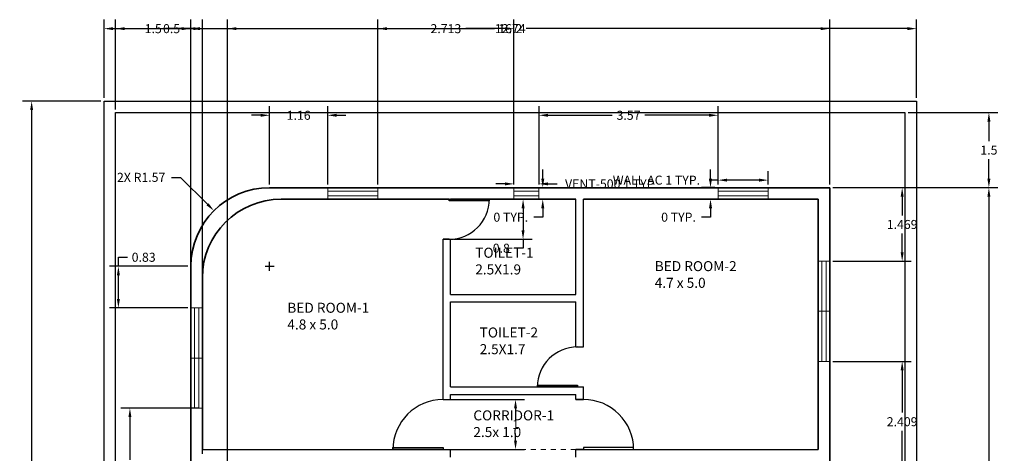
# Model space of a CAD drawing. Units: metres. Extents: x 2527.9 to 2558.5, y 2010.7 to 2033.1.
# Tile 3 of 3: x 2538.9 to 2558.5, y 2024.5 to 2033.1. Entities that reach past the tile are written whole.
import ezdxf

# ---------------------------------------------------------------- set-up
doc = ezdxf.new("R2010")
doc.units = ezdxf.units.M
doc.linetypes.add('ACAD_ISO02W100', pattern=[15, 12, -3])
for name, color, linetype, lineweight in [('A-ANNO-DIMS', 2, 'Continuous', 18), ('A-AREA-IDEN', 180, 'Continuous', 18), ('A-DOOR', 249, 'Continuous', 25), ('A-GLAZ', 249, 'Continuous', 18), ('A-WALL-OVHD', 6, 'ACAD_ISO02W100', 18), ('AC &V', 211, 'Continuous', 18), ('C-SITE-WALL', 110, 'Continuous', 30), ('INNER WALL', 109, 'Continuous', 30), ('OUTER WALL', 110, 'Continuous', 35)]:
    doc.layers.add(name, color=color, linetype=linetype, lineweight=lineweight)
doc.styles.get("Standard").update_dxf_attribs({"font": 'arial.ttf'})
doc.dimstyles.get("Standard").update_dxf_attribs({"dimtxt": 0.18, "dimasz": 0.18, "dimexe": 0.18, "dimexo": 0.0625, "dimgap": 0.09, "dimtad": 0, "dimtih": 1, "dimtoh": 1, "dimdec": 1, "dimzin": 0, "dimdsep": 46, "dimtxsty": 'Standard', "dimcen": 0.09, "dimadec": 0, "dimazin": 0, "dimtfac": 1, "dimtdec": 1, "dimtofl": 0, "dimtmove": 0, "dimatfit": 3, "dimfxl": 1, "dimtolj": 1, "dimtzin": 0, "dimarcsym": 0})

# ---------------------------------------------------------------- blocks, each defined once
blk = doc.blocks.new('*U2')
for p, q in [((0, 0), (0, -6)), ((40, 0), (40, -6))]:
    blk.add_line(p, q)
blk.add_lwpolyline([(0, 0), (0, 40), (1.75, 40), (1.75, 0)], close=True)
blk.add_arc((0, 0), 40, 0, 90)
blk = doc.blocks.new('*U4')
for p, q in [((0, 0), (0, 6)), ((40, 0), (40, 6))]:
    blk.add_line(p, q)
blk.add_lwpolyline([(0, 0), (0, -40), (1.75, -40), (1.75, 0)], close=True)
blk.add_arc((0, 0), 40, 270, 0)
blk = doc.blocks.new('*U3')
for p, q in [((-40, 0), (-40, 6)), ((0, 0), (0, 6))]:
    blk.add_line(p, q)
blk.add_lwpolyline([(0, 0), (0, -40), (-1.75, -40), (-1.75, 0)], close=True)
blk.add_arc((0, 0), 40, 180, 270)
blk = doc.blocks.new('WIN-2000-DOUBLE')
at = {"ltscale": 0.2}
for p, q in [((0, 0.23), (1, 0.23)), ((0, 0), (0, 0.23)), ((1, 0.23), (1, 0)), ((1, 0.23), (2, 0.23)), ((1, 0), (1, 0.23)), ((2, 0.23), (2, 0)), ((0, 0.16), (1, 0.16)), ((1, 0.07), (0, 0.07)), ((1, 0), (0, 0)), ((1, 0.16), (2, 0.16)), ((2, 0.07), (1, 0.07)), ((2, 0), (1, 0))]:
    blk.add_line(p, q, dxfattribs=at)
blk = doc.blocks.new('AC-WALL-1000')
at = {"ltscale": 0.2}
for p, q in [((0, 0.23), (1, 0.23)), ((0, 0), (0, 0.23)), ((1, 0.23), (1, 0)), ((0, 0.16), (1, 0.16)), ((1, 0.07), (0, 0.07)), ((1, 0), (0, 0))]:
    blk.add_line(p, q, dxfattribs=at)
blk = doc.blocks.new('VENT-500')
at = {"ltscale": 0.2}
for p, q in [((0, 0), (0, 0.5)), ((0.23, 0.5), (0, 0.5)), ((0.07, 0), (0.07, 0.5)), ((0.16, 0.5), (0.16, 0)), ((0.23, 0.5), (0.23, 0)), ((0.23, 0), (0, 0))]:
    blk.add_line(p, q, dxfattribs=at)
blk = doc.blocks.new('*D13')
at = {"layer": 'A-ANNO-DIMS', "color": 0, "lineweight": -2, "ltscale": 0.2, "transparency": 16777216}
for p, q in [((2552.796, 2029.847), (2552.796, 2030.115)), ((2553.796, 2029.847), (2553.796, 2030.115)), ((2552.796, 2029.935), (2552.616, 2029.935)), ((2553.616, 2029.935), (2552.976, 2029.935))]:
    blk.add_line(p, q, dxfattribs=at)
at = {"layer": 'A-ANNO-DIMS', "color": 0, "lineweight": -3, "ltscale": 0.2, "transparency": 16777216}
for points in [[(2552.976, 2029.965), (2552.976, 2029.905), (2552.796, 2029.935)], [(2553.616, 2029.965), (2553.616, 2029.905), (2553.796, 2029.935)]]:
    blk.add_solid(points, dxfattribs=at)
at = {"layer": 'Defpoints', "color": 0, "lineweight": -3, "ltscale": 0.2, "transparency": 16777216}
for p in [(2552.796, 2029.935), (2552.796, 2029.785), (2553.796, 2029.785)]:
    blk.add_point(p, dxfattribs=at)
at = {"layer": 'A-ANNO-DIMS', "color": 0, "ltscale": 0.2, "transparency": 16777216, "insert": (2551.567, 2029.935), "char_height": 0.18, "attachment_point": 5}
blk.add_mtext('\\A1;WALL AC 1 TYP.', dxfattribs=at)
blk = doc.blocks.new('*D14')
at = {"layer": 'A-ANNO-DIMS', "color": 0, "lineweight": -2, "ltscale": 0.2, "transparency": 16777216}
for p, q in [((2552.646, 2029.965), (2552.646, 2030.145)), ((2552.734, 2029.785), (2552.466, 2029.785)), ((2552.734, 2029.555), (2552.466, 2029.555)), ((2552.646, 2029.375), (2552.646, 2029.195)), ((2552.646, 2029.195), (2552.466, 2029.195))]:
    blk.add_line(p, q, dxfattribs=at)
at = {"layer": 'A-ANNO-DIMS', "color": 0, "lineweight": -3, "ltscale": 0.2, "transparency": 16777216}
for points in [[(2552.616, 2029.965), (2552.676, 2029.965), (2552.646, 2029.785)], [(2552.616, 2029.375), (2552.676, 2029.375), (2552.646, 2029.555)]]:
    blk.add_solid(points, dxfattribs=at)
at = {"layer": 'Defpoints', "color": 0, "lineweight": -3, "ltscale": 0.2, "transparency": 16777216}
for p in [(2552.796, 2029.785), (2552.646, 2029.555), (2552.796, 2029.555)]:
    blk.add_point(p, dxfattribs=at)
at = {"layer": 'A-ANNO-DIMS', "color": 0, "ltscale": 0.2, "transparency": 16777216, "insert": (2552.008, 2029.195), "char_height": 0.18, "attachment_point": 5}
blk.add_mtext('\\A1;0 TYP.', dxfattribs=at)
blk = doc.blocks.new('*D15')
at = {"layer": 'A-ANNO-DIMS', "color": 0, "lineweight": -2, "ltscale": 0.2, "transparency": 16777216}
for p, q in [((2548.726, 2029.847), (2548.726, 2030.04)), ((2549.226, 2029.847), (2549.226, 2030.04)), ((2548.546, 2029.86), (2548.366, 2029.86)), ((2549.406, 2029.86), (2549.586, 2029.86))]:
    blk.add_line(p, q, dxfattribs=at)
at = {"layer": 'A-ANNO-DIMS', "color": 0, "lineweight": -3, "ltscale": 0.2, "transparency": 16777216}
for points in [[(2548.546, 2029.89), (2548.546, 2029.83), (2548.726, 2029.86)], [(2549.406, 2029.89), (2549.406, 2029.83), (2549.226, 2029.86)]]:
    blk.add_solid(points, dxfattribs=at)
at = {"layer": 'Defpoints', "color": 0, "lineweight": -3, "ltscale": 0.2, "transparency": 16777216}
for p in [(2548.726, 2029.785), (2549.226, 2029.86), (2549.226, 2029.785)]:
    blk.add_point(p, dxfattribs=at)
at = {"layer": 'A-ANNO-DIMS', "color": 0, "ltscale": 0.2, "transparency": 16777216, "insert": (2550.671, 2029.86), "char_height": 0.18, "attachment_point": 5}
blk.add_mtext('\\A1;VENT-500 1 TYP.', dxfattribs=at)
blk = doc.blocks.new('*D16')
at = {"layer": 'A-ANNO-DIMS', "color": 0, "lineweight": -2, "ltscale": 0.2, "transparency": 16777216}
for p, q in [((2549.301, 2029.965), (2549.301, 2030.145)), ((2549.288, 2029.785), (2549.481, 2029.785)), ((2549.288, 2029.555), (2549.481, 2029.555)), ((2549.301, 2029.375), (2549.301, 2029.195)), ((2549.301, 2029.195), (2549.121, 2029.195))]:
    blk.add_line(p, q, dxfattribs=at)
at = {"layer": 'A-ANNO-DIMS', "color": 0, "lineweight": -3, "ltscale": 0.2, "transparency": 16777216}
for points in [[(2549.271, 2029.965), (2549.331, 2029.965), (2549.301, 2029.785)], [(2549.271, 2029.375), (2549.331, 2029.375), (2549.301, 2029.555)]]:
    blk.add_solid(points, dxfattribs=at)
at = {"layer": 'Defpoints', "color": 0, "lineweight": -3, "ltscale": 0.2, "transparency": 16777216}
for p in [(2549.226, 2029.785), (2549.226, 2029.555), (2549.301, 2029.555)]:
    blk.add_point(p, dxfattribs=at)
at = {"layer": 'A-ANNO-DIMS', "color": 0, "ltscale": 0.2, "transparency": 16777216, "insert": (2548.663, 2029.195), "char_height": 0.18, "attachment_point": 5}
blk.add_mtext('\\A1;0 TYP.', dxfattribs=at)
blk = doc.blocks.new('*D17')
at = {"layer": 'A-ANNO-DIMS', "color": 0, "lineweight": -2, "ltscale": 0.2, "transparency": 16777216}
for p, q in [((2540.553, 2031.577), (2540.553, 2033.14)), ((2556.753, 2031.577), (2556.753, 2033.14)), ((2540.733, 2032.96), (2548.339, 2032.96)), ((2556.573, 2032.96), (2548.968, 2032.96))]:
    blk.add_line(p, q, dxfattribs=at)
at = {"layer": 'A-ANNO-DIMS', "color": 0, "lineweight": -3, "ltscale": 0.2, "transparency": 16777216}
for points in [[(2540.733, 2032.99), (2540.733, 2032.93), (2540.553, 2032.96)], [(2556.573, 2032.99), (2556.573, 2032.93), (2556.753, 2032.96)]]:
    blk.add_solid(points, dxfattribs=at)
at = {"layer": 'Defpoints', "color": 0, "lineweight": -3, "ltscale": 0.2, "transparency": 16777216}
for p in [(2556.753, 2032.96), (2540.553, 2031.515), (2556.753, 2031.515)]:
    blk.add_point(p, dxfattribs=at)
at = {"layer": 'A-ANNO-DIMS', "color": 0, "ltscale": 0.2, "transparency": 16777216, "insert": (2548.653, 2032.96), "char_height": 0.18, "attachment_point": 5}
blk.add_mtext('\\A1;16.2', dxfattribs=at)
blk = doc.blocks.new('*D18')
at = {"layer": 'A-ANNO-DIMS', "color": 0, "lineweight": -2, "ltscale": 0.2, "transparency": 16777216}
for p, q in [((2540.491, 2031.515), (2538.928, 2031.515)), ((2539.108, 2031.335), (2539.108, 2022.096)), ((2539.108, 2012.495), (2539.108, 2021.733)), ((2540.491, 2012.315), (2538.928, 2012.315))]:
    blk.add_line(p, q, dxfattribs=at)
at = {"layer": 'A-ANNO-DIMS', "color": 0, "lineweight": -3, "ltscale": 0.2, "transparency": 16777216}
for points in [[(2539.078, 2031.335), (2539.138, 2031.335), (2539.108, 2031.515)], [(2539.078, 2012.495), (2539.138, 2012.495), (2539.108, 2012.315)]]:
    blk.add_solid(points, dxfattribs=at)
at = {"layer": 'Defpoints', "color": 0, "lineweight": -3, "ltscale": 0.2, "transparency": 16777216}
for p in [(2539.108, 2031.515), (2540.553, 2031.515), (2540.553, 2012.315)]:
    blk.add_point(p, dxfattribs=at)
at = {"layer": 'A-ANNO-DIMS', "color": 0, "ltscale": 0.2, "transparency": 16777216, "insert": (2539.108, 2021.915), "char_height": 0.18, "attachment_point": 5}
blk.add_mtext('\\A1;19.2', dxfattribs=at)
blk = doc.blocks.new('*D19')
at = {"layer": 'A-ANNO-DIMS', "color": 0, "lineweight": -2, "ltscale": 0.2, "transparency": 16777216}
for p, q in [((2542.283, 2028.277), (2542.283, 2033.14)), ((2555.023, 2029.847), (2555.023, 2033.14)), ((2542.463, 2032.96), (2548.268, 2032.96)), ((2554.843, 2032.96), (2549.038, 2032.96))]:
    blk.add_line(p, q, dxfattribs=at)
at = {"layer": 'A-ANNO-DIMS', "color": 0, "lineweight": -3, "ltscale": 0.2, "transparency": 16777216}
for points in [[(2542.463, 2032.99), (2542.463, 2032.93), (2542.283, 2032.96)], [(2554.843, 2032.99), (2554.843, 2032.93), (2555.023, 2032.96)]]:
    blk.add_solid(points, dxfattribs=at)
at = {"layer": 'Defpoints', "color": 0, "lineweight": -3, "ltscale": 0.2, "transparency": 16777216}
for p in [(2555.023, 2032.96), (2555.023, 2029.785), (2542.283, 2028.215)]:
    blk.add_point(p, dxfattribs=at)
at = {"layer": 'A-ANNO-DIMS', "color": 0, "ltscale": 0.2, "transparency": 16777216, "insert": (2548.653, 2032.96), "char_height": 0.18, "attachment_point": 5}
blk.add_mtext('\\A1;12.74', dxfattribs=at)
blk = doc.blocks.new('*D20')
at = {"layer": 'A-ANNO-DIMS', "color": 0, "lineweight": -2, "ltscale": 0.2, "transparency": 16777216}
for p, q in [((2555.086, 2029.785), (2558.378, 2029.785)), ((2558.198, 2029.605), (2558.198, 2022.602)), ((2558.198, 2015.235), (2558.198, 2022.238)), ((2555.086, 2015.055), (2558.378, 2015.055))]:
    blk.add_line(p, q, dxfattribs=at)
at = {"layer": 'A-ANNO-DIMS', "color": 0, "lineweight": -3, "ltscale": 0.2, "transparency": 16777216}
for points in [[(2558.168, 2029.605), (2558.228, 2029.605), (2558.198, 2029.785)], [(2558.168, 2015.235), (2558.228, 2015.235), (2558.198, 2015.055)]]:
    blk.add_solid(points, dxfattribs=at)
at = {"layer": 'Defpoints', "color": 0, "lineweight": -3, "ltscale": 0.2, "transparency": 16777216}
for p in [(2555.023, 2029.785), (2558.198, 2029.785), (2555.023, 2015.055)]:
    blk.add_point(p, dxfattribs=at)
at = {"layer": 'A-ANNO-DIMS', "color": 0, "ltscale": 0.2, "transparency": 16777216, "insert": (2558.198, 2022.42), "char_height": 0.18, "attachment_point": 5}
blk.add_mtext('\\A1;14.73', dxfattribs=at)
blk = doc.blocks.new('*D21')
at = {"layer": 'A-ANNO-DIMS', "color": 0, "lineweight": -2, "ltscale": 0.2, "transparency": 16777216}
for p, q in [((2540.783, 2031.347), (2540.783, 2033.14)), ((2542.283, 2028.277), (2542.283, 2033.14)), ((2540.963, 2032.96), (2541.287, 2032.96)), ((2542.103, 2032.96), (2541.779, 2032.96))]:
    blk.add_line(p, q, dxfattribs=at)
at = {"layer": 'A-ANNO-DIMS', "color": 0, "lineweight": -3, "ltscale": 0.2, "transparency": 16777216}
for points in [[(2540.963, 2032.99), (2540.963, 2032.93), (2540.783, 2032.96)], [(2542.103, 2032.99), (2542.103, 2032.93), (2542.283, 2032.96)]]:
    blk.add_solid(points, dxfattribs=at)
at = {"layer": 'Defpoints', "color": 0, "lineweight": -3, "ltscale": 0.2, "transparency": 16777216}
for p in [(2542.283, 2032.96), (2540.783, 2031.285), (2542.283, 2028.215)]:
    blk.add_point(p, dxfattribs=at)
at = {"layer": 'A-ANNO-DIMS', "color": 0, "ltscale": 0.2, "transparency": 16777216, "insert": (2541.533, 2032.96), "char_height": 0.18, "attachment_point": 5}
blk.add_mtext('\\A1;1.5', dxfattribs=at)
blk = doc.blocks.new('*D22')
at = {"layer": 'A-ANNO-DIMS', "color": 0, "lineweight": -2, "ltscale": 0.2, "transparency": 16777216}
for p, q in [((2556.586, 2031.285), (2558.378, 2031.285)), ((2558.198, 2031.105), (2558.198, 2030.716)), ((2558.198, 2029.965), (2558.198, 2030.353)), ((2555.086, 2029.785), (2558.378, 2029.785))]:
    blk.add_line(p, q, dxfattribs=at)
at = {"layer": 'A-ANNO-DIMS', "color": 0, "lineweight": -3, "ltscale": 0.2, "transparency": 16777216}
for points in [[(2558.168, 2031.105), (2558.228, 2031.105), (2558.198, 2031.285)], [(2558.168, 2029.965), (2558.228, 2029.965), (2558.198, 2029.785)]]:
    blk.add_solid(points, dxfattribs=at)
at = {"layer": 'Defpoints', "color": 0, "lineweight": -3, "ltscale": 0.2, "transparency": 16777216}
for p in [(2556.523, 2031.285), (2558.198, 2031.285), (2555.023, 2029.785)]:
    blk.add_point(p, dxfattribs=at)
at = {"layer": 'A-ANNO-DIMS', "color": 0, "ltscale": 0.2, "transparency": 16777216, "insert": (2558.198, 2030.535), "char_height": 0.18, "attachment_point": 5}
blk.add_mtext('\\A1;1.5', dxfattribs=at)
blk = doc.blocks.new('*D50')
at = {"layer": 'A-ANNO-DIMS', "color": 0, "lineweight": -2, "ltscale": 0.2, "transparency": 16777216}
for p, q in [((2543.853, 2029.847), (2543.853, 2031.41)), ((2545.013, 2029.847), (2545.013, 2031.41)), ((2543.673, 2031.23), (2543.493, 2031.23)), ((2545.193, 2031.23), (2545.373, 2031.23))]:
    blk.add_line(p, q, dxfattribs=at)
at = {"layer": 'A-ANNO-DIMS', "color": 0, "lineweight": -3, "ltscale": 0.2, "transparency": 16777216}
for points in [[(2543.673, 2031.26), (2543.673, 2031.2), (2543.853, 2031.23)], [(2545.193, 2031.26), (2545.193, 2031.2), (2545.013, 2031.23)]]:
    blk.add_solid(points, dxfattribs=at)
at = {"layer": 'Defpoints', "color": 0, "lineweight": -3, "ltscale": 0.2, "transparency": 16777216}
for p in [(2545.013, 2031.23), (2543.853, 2029.785), (2545.013, 2029.785)]:
    blk.add_point(p, dxfattribs=at)
at = {"layer": 'A-ANNO-DIMS', "color": 0, "ltscale": 0.2, "transparency": 16777216, "insert": (2544.433, 2031.23), "char_height": 0.18, "attachment_point": 5}
blk.add_mtext('\\A1;1.16', dxfattribs=at)
blk = doc.blocks.new('*D51')
at = {"layer": 'A-ANNO-DIMS', "color": 0, "lineweight": -2, "ltscale": 0.2, "transparency": 16777216}
for p, q in [((2546.013, 2029.847), (2546.013, 2033.14)), ((2548.726, 2029.847), (2548.726, 2033.14)), ((2546.193, 2032.96), (2546.974, 2032.96)), ((2548.546, 2032.96), (2547.765, 2032.96))]:
    blk.add_line(p, q, dxfattribs=at)
at = {"layer": 'A-ANNO-DIMS', "color": 0, "lineweight": -3, "ltscale": 0.2, "transparency": 16777216}
for points in [[(2546.193, 2032.99), (2546.193, 2032.93), (2546.013, 2032.96)], [(2548.546, 2032.99), (2548.546, 2032.93), (2548.726, 2032.96)]]:
    blk.add_solid(points, dxfattribs=at)
at = {"layer": 'Defpoints', "color": 0, "lineweight": -3, "ltscale": 0.2, "transparency": 16777216}
for p in [(2548.726, 2032.96), (2546.013, 2029.785), (2548.726, 2029.785)]:
    blk.add_point(p, dxfattribs=at)
at = {"layer": 'A-ANNO-DIMS', "color": 0, "ltscale": 0.2, "transparency": 16777216, "insert": (2547.369, 2032.96), "char_height": 0.18, "attachment_point": 5}
blk.add_mtext('\\A1;2.713', dxfattribs=at)
blk = doc.blocks.new('*D52')
at = {"layer": 'A-ANNO-DIMS', "color": 0, "lineweight": -2, "ltscale": 0.2, "transparency": 16777216}
for p, q in [((2549.226, 2029.847), (2549.226, 2031.41)), ((2552.796, 2029.847), (2552.796, 2031.41)), ((2549.406, 2031.23), (2550.687, 2031.23)), ((2552.616, 2031.23), (2551.335, 2031.23))]:
    blk.add_line(p, q, dxfattribs=at)
at = {"layer": 'A-ANNO-DIMS', "color": 0, "lineweight": -3, "ltscale": 0.2, "transparency": 16777216}
for points in [[(2549.406, 2031.26), (2549.406, 2031.2), (2549.226, 2031.23)], [(2552.616, 2031.26), (2552.616, 2031.2), (2552.796, 2031.23)]]:
    blk.add_solid(points, dxfattribs=at)
at = {"layer": 'Defpoints', "color": 0, "lineweight": -3, "ltscale": 0.2, "transparency": 16777216}
for p in [(2552.796, 2031.23), (2549.226, 2029.785), (2552.796, 2029.785)]:
    blk.add_point(p, dxfattribs=at)
at = {"layer": 'A-ANNO-DIMS', "color": 0, "ltscale": 0.2, "transparency": 16777216, "insert": (2551.011, 2031.23), "char_height": 0.18, "attachment_point": 5}
blk.add_mtext('\\A1;3.57', dxfattribs=at)
blk = doc.blocks.new('*D53')
at = {"layer": 'A-ANNO-DIMS', "color": 0, "lineweight": -2, "ltscale": 0.2, "transparency": 16777216}
for p, q in [((2555.086, 2029.785), (2556.648, 2029.785)), ((2556.468, 2029.605), (2556.468, 2029.232)), ((2556.468, 2028.496), (2556.468, 2028.868)), ((2555.086, 2028.316), (2556.648, 2028.316))]:
    blk.add_line(p, q, dxfattribs=at)
at = {"layer": 'A-ANNO-DIMS', "color": 0, "lineweight": -3, "ltscale": 0.2, "transparency": 16777216}
for points in [[(2556.438, 2029.605), (2556.498, 2029.605), (2556.468, 2029.785)], [(2556.438, 2028.496), (2556.498, 2028.496), (2556.468, 2028.316)]]:
    blk.add_solid(points, dxfattribs=at)
at = {"layer": 'Defpoints', "color": 0, "lineweight": -3, "ltscale": 0.2, "transparency": 16777216}
for p in [(2555.023, 2029.785), (2555.023, 2028.316), (2556.468, 2028.316)]:
    blk.add_point(p, dxfattribs=at)
at = {"layer": 'A-ANNO-DIMS', "color": 0, "ltscale": 0.2, "transparency": 16777216, "insert": (2556.468, 2029.05), "char_height": 0.18, "attachment_point": 5}
blk.add_mtext('\\A1;1.469', dxfattribs=at)
blk = doc.blocks.new('*D54')
at = {"layer": 'A-ANNO-DIMS', "color": 0, "lineweight": -2, "ltscale": 0.2, "transparency": 16777216}
for p, q in [((2555.086, 2026.316), (2556.648, 2026.316)), ((2556.468, 2026.136), (2556.468, 2025.293)), ((2556.468, 2024.087), (2556.468, 2024.929)), ((2555.086, 2023.907), (2556.648, 2023.907))]:
    blk.add_line(p, q, dxfattribs=at)
at = {"layer": 'A-ANNO-DIMS', "color": 0, "lineweight": -3, "ltscale": 0.2, "transparency": 16777216}
for points in [[(2556.438, 2026.136), (2556.498, 2026.136), (2556.468, 2026.316)], [(2556.438, 2024.087), (2556.498, 2024.087), (2556.468, 2023.907)]]:
    blk.add_solid(points, dxfattribs=at)
at = {"layer": 'Defpoints', "color": 0, "lineweight": -3, "ltscale": 0.2, "transparency": 16777216}
for p in [(2555.023, 2026.316), (2555.023, 2023.907), (2556.468, 2023.907)]:
    blk.add_point(p, dxfattribs=at)
at = {"layer": 'A-ANNO-DIMS', "color": 0, "ltscale": 0.2, "transparency": 16777216, "insert": (2556.468, 2025.111), "char_height": 0.18, "attachment_point": 5}
blk.add_mtext('\\A1;2.409', dxfattribs=at)
blk = doc.blocks.new('*D57')
at = {"layer": 'A-ANNO-DIMS', "color": 0, "lineweight": -2, "ltscale": 0.2, "transparency": 16777216}
for p, q in [((2540.838, 2028.215), (2540.838, 2028.395)), ((2540.838, 2028.395), (2541.018, 2028.395)), ((2542.221, 2028.215), (2540.658, 2028.215)), ((2540.838, 2027.563), (2540.838, 2028.035)), ((2542.221, 2027.383), (2540.658, 2027.383))]:
    blk.add_line(p, q, dxfattribs=at)
at = {"layer": 'A-ANNO-DIMS', "color": 0, "lineweight": -3, "ltscale": 0.2, "transparency": 16777216}
for points in [[(2540.808, 2028.035), (2540.868, 2028.035), (2540.838, 2028.215)], [(2540.808, 2027.563), (2540.868, 2027.563), (2540.838, 2027.383)]]:
    blk.add_solid(points, dxfattribs=at)
at = {"layer": 'Defpoints', "color": 0, "lineweight": -3, "ltscale": 0.2, "transparency": 16777216}
for p in [(2540.838, 2028.215), (2542.283, 2028.215), (2542.283, 2027.383)]:
    blk.add_point(p, dxfattribs=at)
at = {"layer": 'A-ANNO-DIMS', "color": 0, "ltscale": 0.2, "transparency": 16777216, "insert": (2541.342, 2028.395), "char_height": 0.18, "attachment_point": 5}
blk.add_mtext('\\A1;0.83', dxfattribs=at)
blk = doc.blocks.new('*D58')
at = {"layer": 'A-ANNO-DIMS', "color": 0, "lineweight": -2, "ltscale": 0.2, "transparency": 16777216}
for p, q in [((2542.451, 2025.383), (2540.888, 2025.383)), ((2541.068, 2025.203), (2541.068, 2024.351)), ((2541.068, 2023.139), (2541.068, 2023.991)), ((2542.451, 2022.959), (2540.888, 2022.959))]:
    blk.add_line(p, q, dxfattribs=at)
at = {"layer": 'A-ANNO-DIMS', "color": 0, "lineweight": -3, "ltscale": 0.2, "transparency": 16777216}
for points in [[(2541.038, 2025.203), (2541.098, 2025.203), (2541.068, 2025.383)], [(2541.038, 2023.139), (2541.098, 2023.139), (2541.068, 2022.959)]]:
    blk.add_solid(points, dxfattribs=at)
at = {"layer": 'Defpoints', "color": 0, "lineweight": -3, "ltscale": 0.2, "transparency": 16777216}
for p in [(2541.068, 2025.383), (2542.513, 2025.383), (2542.513, 2022.959)]:
    blk.add_point(p, dxfattribs=at)
at = {"layer": 'A-ANNO-DIMS', "color": 0, "ltscale": 0.2, "transparency": 16777216, "insert": (2541.068, 2024.171), "char_height": 0.18, "attachment_point": 5}
blk.add_mtext('\\A1;2.42', dxfattribs=at)
blk = doc.blocks.new('*D63')
at = {"layer": 'A-ANNO-DIMS', "color": 0, "lineweight": -2, "ltscale": 0.2, "transparency": 16777216}
for p, q in [((2547.376, 2025.555), (2548.938, 2025.555)), ((2548.758, 2025.375), (2548.758, 2025.235)), ((2548.758, 2024.735), (2548.758, 2024.874)), ((2547.376, 2024.555), (2548.938, 2024.555))]:
    blk.add_line(p, q, dxfattribs=at)
at = {"layer": 'A-ANNO-DIMS', "color": 0, "lineweight": -3, "ltscale": 0.2, "transparency": 16777216}
for points in [[(2548.728, 2025.375), (2548.788, 2025.375), (2548.758, 2025.555)], [(2548.728, 2024.735), (2548.788, 2024.735), (2548.758, 2024.555)]]:
    blk.add_solid(points, dxfattribs=at)
at = {"layer": 'Defpoints', "color": 0, "lineweight": -3, "ltscale": 0.2, "transparency": 16777216}
for p in [(2547.313, 2025.555), (2547.313, 2024.555), (2548.758, 2024.555)]:
    blk.add_point(p, dxfattribs=at)
at = {"layer": 'A-ANNO-DIMS', "color": 0, "ltscale": 0.2, "transparency": 16777216, "insert": (2548.758, 2025.055), "char_height": 0.18, "attachment_point": 5}
blk.add_mtext('\\A1;1', dxfattribs=at)
blk = doc.blocks.new('*D64')
at = {"layer": 'A-ANNO-DIMS', "color": 0, "lineweight": -2, "ltscale": 0.2, "transparency": 16777216}
for p, q in [((2547.526, 2029.555), (2549.088, 2029.555)), ((2548.908, 2029.375), (2548.908, 2028.935)), ((2547.526, 2028.755), (2549.088, 2028.755)), ((2548.908, 2028.755), (2548.908, 2028.575)), ((2548.908, 2028.575), (2548.728, 2028.575))]:
    blk.add_line(p, q, dxfattribs=at)
at = {"layer": 'A-ANNO-DIMS', "color": 0, "lineweight": -3, "ltscale": 0.2, "transparency": 16777216}
for points in [[(2548.878, 2029.375), (2548.938, 2029.375), (2548.908, 2029.555)], [(2548.878, 2028.935), (2548.938, 2028.935), (2548.908, 2028.755)]]:
    blk.add_solid(points, dxfattribs=at)
at = {"layer": 'Defpoints', "color": 0, "lineweight": -3, "ltscale": 0.2, "transparency": 16777216}
for p in [(2547.463, 2029.555), (2547.463, 2028.755), (2548.908, 2028.755)]:
    blk.add_point(p, dxfattribs=at)
at = {"layer": 'A-ANNO-DIMS', "color": 0, "ltscale": 0.2, "transparency": 16777216, "insert": (2548.474, 2028.575), "char_height": 0.18, "attachment_point": 5}
blk.add_mtext('\\A1;0.8', dxfattribs=at)
blk = doc.blocks.new('*D65')
at = {"layer": 'A-ANNO-DIMS', "color": 0, "lineweight": -2, "ltscale": 0.2, "transparency": 16777216}
for p, q in [((2542.513, 2024.467), (2542.513, 2033.14)), ((2543.013, 2023.967), (2543.013, 2033.14)), ((2542.333, 2032.96), (2542.153, 2032.96)), ((2543.193, 2032.96), (2543.373, 2032.96))]:
    blk.add_line(p, q, dxfattribs=at)
at = {"layer": 'A-ANNO-DIMS', "color": 0, "lineweight": -3, "ltscale": 0.2, "transparency": 16777216}
for points in [[(2542.333, 2032.99), (2542.333, 2032.93), (2542.513, 2032.96)], [(2543.193, 2032.99), (2543.193, 2032.93), (2543.013, 2032.96)]]:
    blk.add_solid(points, dxfattribs=at)
at = {"layer": 'Defpoints', "color": 0, "lineweight": -3, "ltscale": 0.2, "transparency": 16777216}
for p in [(2542.513, 2032.96), (2542.513, 2024.405), (2543.013, 2023.905)]:
    blk.add_point(p, dxfattribs=at)
at = {"layer": 'A-ANNO-DIMS', "color": 0, "ltscale": 0.2, "transparency": 16777216, "insert": (2541.899, 2032.96), "char_height": 0.18, "attachment_point": 5}
blk.add_mtext('\\A1;0.5', dxfattribs=at)
blk = doc.blocks.new('*D66')
at = {"layer": 'A-ANNO-DIMS', "color": 0, "lineweight": -2, "ltscale": 0.2, "transparency": 16777216}
for p, q in [((2541.897, 2029.991), (2542.077, 2029.991)), ((2542.077, 2029.991), (2542.616, 2029.452)), ((2543.763, 2028.215), (2543.943, 2028.215)), ((2543.853, 2028.125), (2543.853, 2028.305))]:
    blk.add_line(p, q, dxfattribs=at)
at = {"layer": 'A-ANNO-DIMS', "color": 0, "lineweight": -3, "ltscale": 0.2, "transparency": 16777216}
blk.add_solid([(2542.637, 2029.473), (2542.595, 2029.431), (2542.743, 2029.325)], dxfattribs=at)
at = {"layer": 'Defpoints', "color": 0, "lineweight": -3, "ltscale": 0.2, "transparency": 16777216}
for p in [(2542.743, 2029.325), (2543.853, 2028.215)]:
    blk.add_point(p, dxfattribs=at)
at = {"layer": 'A-ANNO-DIMS', "color": 0, "ltscale": 0.2, "transparency": 16777216, "insert": (2541.292, 2029.991), "char_height": 0.18, "attachment_point": 5}
blk.add_mtext('\\A1;2X R1.57', dxfattribs=at)

msp = doc.modelspace()

# ---------------------------------------------------------------- linework, layer by layer
at = {"layer": 'A-WALL-OVHD', "ltscale": 0.002}
msp.add_line((2547.4633, 2024.5545), (2549.9633, 2024.5545), dxfattribs=at)
at = {"layer": 'C-SITE-WALL'}
for p, q in [((2540.5533, 2031.5145), (2556.7533, 2031.5145)), ((2540.7833, 2031.2845), (2556.5233, 2031.2845))]:
    msp.add_line(p, q, dxfattribs=at)
for points in [[(2548.0644, 2012.3145), (2540.5533, 2012.3145), (2540.5533, 2031.5145)], [(2556.7533, 2031.5145), (2556.7533, 2012.3145), (2551.0644, 2012.3145)], [(2548.0644, 2012.5445), (2540.7833, 2012.5445), (2540.7833, 2031.2845)], [(2556.5233, 2031.2845), (2556.5233, 2012.5445), (2551.0644, 2012.5445)]]:
    msp.add_lwpolyline(points, dxfattribs=at)
at = {"layer": 'INNER WALL'}
for p, q in [((2547.3133, 2029.5545), (2547.4633, 2029.5545)), ((2549.9633, 2027.6545), (2549.9633, 2029.5545)), ((2550.1133, 2026.6045), (2550.1133, 2029.5545)), ((2547.3133, 2028.7545), (2547.4633, 2028.7545)), ((2547.3133, 2025.5545), (2547.3133, 2028.7545)), ((2547.4633, 2027.6545), (2547.4633, 2028.7545)), ((2547.4633, 2027.6545), (2549.9633, 2027.6545)), ((2547.4633, 2027.5045), (2549.9633, 2027.5045)), ((2547.4633, 2025.8045), (2547.4633, 2027.5045)), ((2549.9633, 2026.6045), (2549.9633, 2027.5045)), ((2549.9633, 2026.6045), (2550.1133, 2026.6045)), ((2547.4633, 2025.8045), (2549.9633, 2025.8045)), ((2549.9633, 2025.8045), (2550.1133, 2025.8045)), ((2550.1133, 2025.5545), (2550.1133, 2025.8045)), ((2547.4633, 2025.6545), (2549.9633, 2025.6545)), ((2547.4633, 2025.5545), (2547.4633, 2025.6545)), ((2549.9633, 2025.5545), (2549.9633, 2025.6545)), ((2549.9633, 2025.5545), (2549.9633, 2025.6545)), ((2547.3133, 2025.5545), (2547.4633, 2025.5545)), ((2549.9633, 2025.5545), (2550.1133, 2025.5545)), ((2542.5133, 2024.5545), (2547.3133, 2024.5545)), ((2547.3133, 2024.5545), (2547.4633, 2024.5545)), ((2547.4633, 2024.4045), (2547.4633, 2024.5545)), ((2549.9633, 2024.5545), (2550.1133, 2024.5545)), ((2549.9633, 2024.4045), (2549.9633, 2024.5545)), ((2550.1133, 2024.5545), (2554.7933, 2024.5545))]:
    msp.add_line(p, q, dxfattribs=at)
at = {"layer": 'OUTER WALL'}
for p, q in [((2543.8533, 2029.7845), (2555.0233, 2029.7845)), ((2555.0233, 2029.7845), (2555.0233, 2015.0545)), ((2544.0833, 2029.5545), (2547.3133, 2029.5545)), ((2547.4633, 2029.5545), (2549.9633, 2029.5545)), ((2550.1133, 2029.5545), (2554.7933, 2029.5545)), ((2554.7933, 2029.5545), (2554.7933, 2024.5545)), ((2542.2833, 2015.5245), (2542.2833, 2028.2145)), ((2542.5133, 2024.5545), (2542.5133, 2027.9845))]:
    msp.add_line(p, q, dxfattribs=at)
for centre in [(2543.8533, 2028.2145), (2544.0833, 2027.9845)]:
    msp.add_arc(centre, 1.57, 90, 180, dxfattribs=at)

# ---------------------------------------------------------------- block references
at = {"layer": 'A-DOOR'}
for name, p, xscale, yscale, zscale, rotation in [('*U2', (2547.4333, 2029.5545), 0.0199999999999985, 0.0199999999999985, 0.0199999999999985, 270), ('*U2', (2549.9933, 2025.8045), 0.0199999999999985, 0.0199999999999985, 0.0199999999999985, 89.99999999999999), ('*U3', (2547.3133, 2024.5545), 0.0249999999999996, 0.0249999999999996, 0.0249999999999996, 270), ('*U4', (2550.1133, 2024.5545), 0.0249999999999996, 0.0249999999999996, 0.0249999999999996, 89.99999999999999)]:
    msp.add_blockref(name, p, dxfattribs=dict(at, xscale=xscale, yscale=yscale, zscale=zscale, rotation=rotation))
at = {"layer": 'A-GLAZ'}
for p, rotation in [((2555.0233, 2026.3157), 89.99999999998612), ((2542.5133, 2025.3831), 90.00000000002422)]:
    msp.add_blockref('WIN-2000-DOUBLE', p, dxfattribs=dict(at, rotation=rotation))
at = {"layer": 'AC &V'}
msp.add_blockref('AC-WALL-1000', (2545.0129, 2029.5545), dxfattribs=at)
for name, p, rotation in [('VENT-500', (2548.7258, 2029.7845), 270.0000000002778), ('AC-WALL-1000', (2553.7962, 2029.7845), 180)]:
    msp.add_blockref(name, p, dxfattribs=dict(at, rotation=rotation))

# ---------------------------------------------------------------- texts
at = {"layer": 'A-AREA-IDEN', "char_height": 0.2, "attachment_point": 1}
for s, width, insert in [('TOILET-1 2.5X1.9', 1.31727, (2547.9548, 2028.5853)), ('BED ROOM-2   4.7 x 5.0', 1.785754, (2551.5337, 2028.3176)), ('BED ROOM-1   4.8 x 5.0', 1.809794, (2544.2069, 2027.4863)), ('TOILET-2 2.5X1.7', 1.31727, (2548.0427, 2026.9929)), ('CORRIDOR-1   2.5x 1.0', 1.770765, (2547.9162, 2025.3377))]:
    msp.add_mtext_dynamic_manual_height_columns(s, width=width, gutter_width=12.5, heights=[0], dxfattribs=dict(at, insert=insert))

# ---------------------------------------------------------------- dimensions: what is measured, and where the dimension line sits
at = {"layer": 'A-ANNO-DIMS', "ltscale": 0.2}
for base, p1, p2, override, picture, middle in [((2556.7533, 2032.9595), (2540.5533, 2031.5145), (2556.7533, 2031.5145), {"dimdec": 1, "dimlfac": 1, "dimrnd": 0, "dimzin": 0, "dimdsep": 46, "dimlunit": 2}, '*D17', (2548.6533, 2032.9595)), ((2542.2833, 2032.9595), (2540.7833, 2031.2845), (2542.2833, 2028.2145), {"dimdec": 1, "dimlfac": 1, "dimrnd": 0, "dimzin": 0, "dimdsep": 46, "dimlunit": 2}, '*D21', (2541.5333, 2032.9595)), ((2542.5133, 2032.9595), (2543.0133, 2023.9045), (2542.5133, 2024.4045), {"dimdec": 1, "dimlfac": 1, "dimrnd": 0, "dimzin": 0, "dimdsep": 46, "dimlunit": 2}, '*D65', (2541.8988, 2032.9595)), ((2555.0233, 2032.9595), (2542.2833, 2028.2145), (2555.0233, 2029.7845), {"dimdec": 2, "dimlfac": 1, "dimrnd": 0, "dimzin": 0, "dimdsep": 46, "dimlunit": 2}, '*D19', (2548.6533, 2032.9595)), ((2548.7258, 2032.9595), (2546.0129, 2029.7845), (2548.7258, 2029.7845), {"dimdec": 3, "dimlfac": 1, "dimrnd": 0, "dimzin": 0, "dimdsep": 46, "dimlunit": 2}, '*D51', (2547.3693, 2032.9595)), ((2545.0129, 2031.2295), (2543.8533, 2029.7845), (2545.0129, 2029.7845), {"dimdec": 2, "dimlfac": 1, "dimrnd": 0, "dimzin": 0, "dimdsep": 46, "dimlunit": 2}, '*D50', (2544.4331, 2031.2295)), ((2552.7962, 2031.2295), (2549.2258, 2029.7845), (2552.7962, 2029.7845), {"dimdec": 2, "dimlfac": 1, "dimrnd": 0, "dimzin": 0, "dimdsep": 46, "dimlunit": 2}, '*D52', (2551.011, 2031.2295))]:
    dim = msp.add_linear_dim(base=base, p1=p1, p2=p2, dimstyle='Standard', override=override, dxfattribs=at)
    dim.commit()
    dim.dimension.update_dxf_attribs({"geometry": picture, "text_midpoint": middle})
for base, p1, p2, angle, override, picture, middle in [((2539.1083, 2031.5145), (2540.5533, 2012.3145), (2540.5533, 2031.5145), 90, {"dimdec": 1, "dimlfac": 1, "dimrnd": 0, "dimzin": 0, "dimdsep": 46, "dimlunit": 2}, '*D18', (2539.1083, 2021.9145)), ((2558.1983, 2031.2845), (2555.0233, 2029.7845), (2556.5233, 2031.2845), 90, {"dimdec": 1, "dimlfac": 1, "dimrnd": 0, "dimzin": 0, "dimdsep": 46, "dimlunit": 2}, '*D22', (2558.1983, 2030.5345)), ((2558.1983, 2029.7845), (2555.0233, 2015.0545), (2555.0233, 2029.7845), 90, {"dimdec": 2, "dimlfac": 1, "dimrnd": 0, "dimzin": 0, "dimdsep": 46, "dimlunit": 2}, '*D20', (2558.1983, 2022.4195)), ((2556.4683, 2028.3157), (2555.0233, 2029.7845), (2555.0233, 2028.3157), 270, {"dimdec": 3, "dimlfac": 1, "dimrnd": 0, "dimzin": 0, "dimdsep": 46, "dimlunit": 2}, '*D53', (2556.4683, 2029.0501)), ((2548.9083, 2028.7545), (2547.4633, 2029.5545), (2547.4633, 2028.7545), 270, {"dimdec": 1, "dimlfac": 1, "dimrnd": 0, "dimzin": 0, "dimdsep": 46, "dimlunit": 2}, '*D64', (2548.4743, 2028.5745)), ((2540.8383, 2028.2145), (2542.2833, 2027.3831), (2542.2833, 2028.2145), 90, {"dimdec": 2, "dimlfac": 1, "dimrnd": 0, "dimzin": 0, "dimdsep": 46, "dimlunit": 2}, '*D57', (2541.3421, 2028.3945)), ((2556.4683, 2023.9067), (2555.0233, 2026.3157), (2555.0233, 2023.9067), 270, {"dimdec": 3, "dimlfac": 1, "dimrnd": 0, "dimzin": 0, "dimdsep": 46, "dimlunit": 2}, '*D54', (2556.4683, 2025.1112)), ((2541.0683, 2025.3831), (2542.5133, 2022.9587), (2542.5133, 2025.3831), 90, {"dimdec": 2, "dimlfac": 1, "dimrnd": 0, "dimzin": 0, "dimdsep": 46, "dimlunit": 2}, '*D58', (2541.0683, 2024.1709)), ((2548.7583, 2024.5545), (2547.3133, 2025.5545), (2547.3133, 2024.5545), 270, {"dimdec": 0, "dimlfac": 1, "dimrnd": 0, "dimzin": 0, "dimdsep": 46, "dimlunit": 2}, '*D63', (2548.7583, 2025.0545))]:
    dim = msp.add_linear_dim(base=base, p1=p1, p2=p2, angle=angle, dimstyle='Standard', override=override, dxfattribs=at)
    dim.commit()
    dim.dimension.update_dxf_attribs({"geometry": picture, "text_midpoint": middle})
for base, p1, p2, angle, text, picture, middle in [((2552.7962, 2029.9345), (2553.7962, 2029.7845), (2552.7962, 2029.7845), 180, 'WALL AC <> TYP.', '*D13', (2551.5675, 2029.9345)), ((2549.3008, 2029.5545), (2549.2258, 2029.7845), (2549.2258, 2029.5545), 270, '<> TYP.', '*D16', (2548.6626, 2029.1945)), ((2549.225797603, 2029.8595364126), (2548.725797603, 2029.7845364126), (2549.225797603, 2029.7845364126), 0.0000000003, 'VENT-500 <> TYP.', '*D15', (2550.6705247517, 2029.8595364126)), ((2552.6462, 2029.5545), (2552.7962, 2029.7845), (2552.7962, 2029.5545), 270, '<> TYP.', '*D14', (2552.008, 2029.1945))]:
    dim = msp.add_linear_dim(base=base, p1=p1, p2=p2, angle=angle, text=text, dimstyle='Standard', override={"dimdec": 0, "dimlfac": 1, "dimrnd": 0, "dimzin": 0, "dimdsep": 46, "dimlunit": 2}, dxfattribs=at)
    dim.commit()
    dim.dimension.update_dxf_attribs({"geometry": picture, "text_midpoint": middle})
dim = msp.add_radius_dim(center=(2543.8533, 2028.2145), mpoint=(2542.7432, 2029.3248), text='2X <>', dimstyle='Standard', override={"dimdec": 2, "dimlfac": 1, "dimrnd": 0, "dimzin": 0, "dimdsep": 46, "dimlunit": 2}, dxfattribs=at)
dim.commit()
dim.dimension.update_dxf_attribs({"geometry": '*D66', "text_midpoint": (2541.2924, 2029.9909), "dimtype": 164})

doc.saveas('drawing.dxf')
